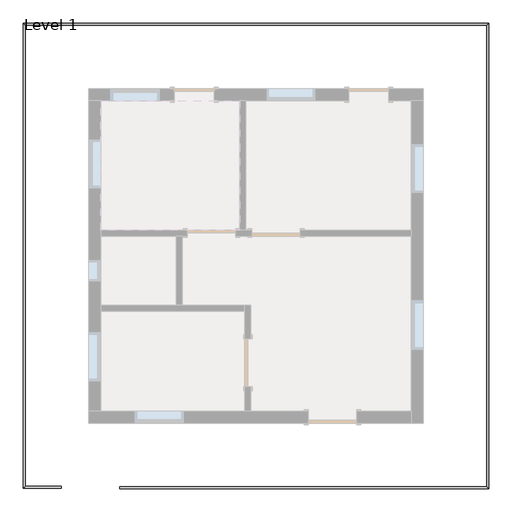
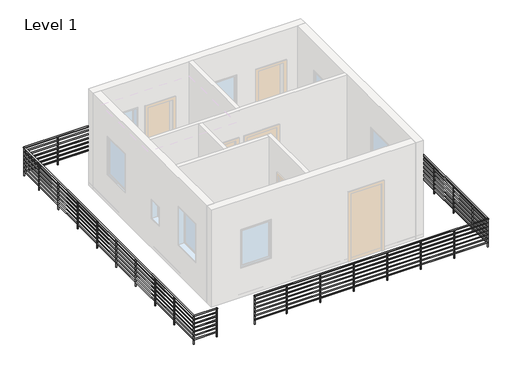
# One storey, part 2 of 2: 1 railing.
"""IFC4 building model written with IfcOpenShell, lengths in millimetres."""

from ifc_helpers import new_model, si_unit, point, frame, frame_2d, origin, origin_with_axes, place, context, project, spatial, circle_curve, ellipse_curve, trimmed, segment, composite_curve, outline, extrude, element, save
from ifc_brep_helpers import plane_surface, cylinder_surface, advanced_brep

model = new_model("IFC4")

# Units and contexts
model_context = context("Model", 3, world=origin())
ifc_project = project(units=[si_unit("LENGTHUNIT", "METRE", prefix="MILLI")], contexts=[model_context])

# Site, building, storey
site = spatial("IfcSite", under=ifc_project)
building = spatial("IfcBuilding", under=site)
storey = spatial("IfcBuildingStorey", under=building, Name="Level 1", Elevation=0.0)

# Railing
placement = place(None, origin())
element("IfcRailing", 1, ObjectType="900mm Pipe", at=placement, inside=storey, context=model_context, shape_type="SolidModel", body=[
    advanced_brep(
    [(-15823.6523905, -4811.14356, 880.0), (-15823.6523905, -4851.14356, 880.0), (-16499.9443193, -4811.14356, 880.0), (-16539.9443193, -4851.14356, 880.0), (-16499.9443193, 3906.0356469, 880.0), (-16539.9443193, 3946.0356469, 880.0), (-7776.9443193, 3906.0356469, 880.0), (-7736.9443193, 3946.0356469, 880.0), (-7776.9443193, -4816.9643531, 880.0), (-7736.9443193, -4856.9643531, 880.0), (-14716.5443193, -4816.9643531, 880.0), (-14716.5443193, -4856.9643531, 880.0)],
    [
        (0, 1, circle_curve(frame((-15823.6523905, -4831.14356, 880.0), z_axis=(1.0, 0.0, 0.0), x_axis=(0.0, -1.0, 0.0)), 20.0)),
        (1, 0, circle_curve(frame((-15823.6523905, -4831.14356, 880.0), z_axis=(1.0, 0.0, 0.0), x_axis=(0.0, -1.0, 0.0)), 20.0)),
        (0, 2),
        (2, 3, ellipse_curve(frame((-16519.9443193, -4831.14356, 880.0), z_axis=(0.7071067811865458, -0.7071067811865492, 0.0), x_axis=(0.7071067811865492, 0.7071067811865458, 0.0)), 28.2842712, 20.0)),
        (3, 1),
        (3, 2, ellipse_curve(frame((-16519.9443193, -4831.14356, 880.0), z_axis=(0.7071067811865458, -0.7071067811865492, 0.0), x_axis=(0.7071067811865492, 0.7071067811865458, 0.0)), 28.2842712, 20.0)),
        (2, 4),
        (4, 5, ellipse_curve(frame((-16519.9443193, 3926.0356469, 880.0), z_axis=(-0.7071067811865493, -0.7071067811865457, 0.0), x_axis=(0.7071067811865457, -0.7071067811865495, 0.0)), 28.2842712, 20.0)),
        (5, 3),
        (5, 4, ellipse_curve(frame((-16519.9443193, 3926.0356469, 880.0), z_axis=(-0.7071067811865493, -0.7071067811865457, 0.0), x_axis=(0.7071067811865457, -0.7071067811865495, 0.0)), 28.2842712, 20.0)),
        (4, 6),
        (6, 7, ellipse_curve(frame((-7756.9443193, 3926.0356469, 880.0), z_axis=(-0.7071067811865446, 0.7071067811865505, 0.0), x_axis=(-0.7071067811865505, -0.7071067811865445, 0.0)), 28.2842712, 20.0)),
        (7, 5),
        (7, 6, ellipse_curve(frame((-7756.9443193, 3926.0356469, 880.0), z_axis=(-0.7071067811865446, 0.7071067811865505, 0.0), x_axis=(-0.7071067811865505, -0.7071067811865445, 0.0)), 28.2842712, 20.0)),
        (6, 8),
        (8, 9, ellipse_curve(frame((-7756.9443193, -4836.9643531, 880.0), z_axis=(0.7071067811865505, 0.7071067811865446, 0.0), x_axis=(-0.7071067811865446, 0.7071067811865503, 0.0)), 28.2842712, 20.0)),
        (9, 7),
        (9, 8, ellipse_curve(frame((-7756.9443193, -4836.9643531, 880.0), z_axis=(0.7071067811865505, 0.7071067811865446, 0.0), x_axis=(-0.7071067811865446, 0.7071067811865503, 0.0)), 28.2842712, 20.0)),
        (10, 11, circle_curve(frame((-14716.5443193, -4836.9643531, 880.0), z_axis=(-1.0, 0.0, 0.0), x_axis=(0.0, -1.0, 0.0)), 20.0)),
        (11, 10, circle_curve(frame((-14716.5443193, -4836.9643531, 880.0), z_axis=(-1.0, 0.0, 0.0), x_axis=(0.0, -1.0, 0.0)), 20.0)),
        (8, 10),
        (11, 9),
    ],
    [
        plane_surface(frame((-15823.6523905, -4831.14356, 900.0), z_axis=(1.0, 0.0, 0.0), x_axis=(0.0, -1.0, 0.0))),
        cylinder_surface(frame((-15823.6523905, -4831.14356, 880.0), z_axis=(1.0, 0.0, 0.0), x_axis=(0.0, -1.0, 0.0)), 20.0),
        cylinder_surface(frame((-16519.9443193, -4831.14356, 880.0), z_axis=(0.0, -1.0, 0.0), x_axis=(-1.0, 0.0, 0.0)), 20.0),
        cylinder_surface(frame((-16519.9443193, 3926.0356469, 880.0), z_axis=(-1.0, 0.0, 0.0), x_axis=(0.0, 1.0, 0.0)), 20.0),
        cylinder_surface(frame((-7756.9443193, 3926.0356469, 880.0), z_axis=(0.0, 1.0, 0.0), x_axis=(1.0, 0.0, 0.0)), 20.0),
        plane_surface(frame((-14716.5443193, -4836.9643531, 900.0), z_axis=(-1.0, 0.0, 0.0), x_axis=(0.0, -1.0, 0.0))),
        cylinder_surface(frame((-7756.9443193, -4836.9643531, 880.0), z_axis=(1.0, 0.0, 0.0), x_axis=(0.0, -1.0, 0.0)), 20.0),
    ],
    [
        (0, [[1, 2]]),
        (1, [[-1, 3, 4, 5]]),
        (1, [[-2, -5, 6, -3]]),
        (2, [[-4, 7, 8, 9]]),
        (2, [[-6, -9, 10, -7]]),
        (3, [[-8, 11, 12, 13]]),
        (3, [[-10, -13, 14, -11]]),
        (4, [[-12, 15, 16, 17]]),
        (4, [[-14, -17, 18, -15]]),
        (5, [[19, 20]]),
        (6, [[-16, 21, -20, 22]]),
        (6, [[-18, -22, -19, -21]]),
    ],
),
    advanced_brep(
    [(-15823.6523905, -4846.14356, 760.0), (-15823.6523905, -4816.14356, 760.0), (-16534.9443193, -4846.14356, 760.0), (-16504.9443193, -4816.14356, 760.0), (-16534.9443193, 3941.0356469, 760.0), (-16504.9443193, 3911.0356469, 760.0), (-7741.9443193, 3941.0356469, 760.0), (-7771.9443193, 3911.0356469, 760.0), (-7741.9443193, -4851.9643531, 760.0), (-7771.9443193, -4821.9643531, 760.0), (-14716.5443193, -4851.9643531, 760.0), (-14716.5443193, -4821.9643531, 760.0)],
    [
        (0, 1, circle_curve(frame((-15823.6523905, -4831.14356, 760.0), z_axis=(1.0, 0.0, 0.0), x_axis=(0.0, 1.0, 0.0)), 15.0)),
        (1, 0, circle_curve(frame((-15823.6523905, -4831.14356, 760.0), z_axis=(1.0, 0.0, 0.0), x_axis=(0.0, 1.0, 0.0)), 15.0)),
        (0, 2),
        (2, 3, ellipse_curve(frame((-16519.9443193, -4831.14356, 760.0), z_axis=(0.7071067811865458, -0.7071067811865492, 0.0), x_axis=(0.7071067811865492, 0.7071067811865458, 0.0)), 21.2132034, 15.0)),
        (3, 1),
        (3, 2, ellipse_curve(frame((-16519.9443193, -4831.14356, 760.0), z_axis=(0.7071067811865458, -0.7071067811865492, 0.0), x_axis=(0.7071067811865492, 0.7071067811865458, 0.0)), 21.2132034, 15.0)),
        (2, 4),
        (4, 5, ellipse_curve(frame((-16519.9443193, 3926.0356469, 760.0), z_axis=(-0.7071067811865493, -0.7071067811865457, 0.0), x_axis=(0.7071067811865457, -0.7071067811865495, 0.0)), 21.2132034, 15.0)),
        (5, 3),
        (5, 4, ellipse_curve(frame((-16519.9443193, 3926.0356469, 760.0), z_axis=(-0.7071067811865493, -0.7071067811865457, 0.0), x_axis=(0.7071067811865457, -0.7071067811865495, 0.0)), 21.2132034, 15.0)),
        (4, 6),
        (6, 7, ellipse_curve(frame((-7756.9443193, 3926.0356469, 760.0), z_axis=(-0.7071067811865446, 0.7071067811865505, 0.0), x_axis=(-0.7071067811865505, -0.7071067811865445, 0.0)), 21.2132034, 15.0)),
        (7, 5),
        (7, 6, ellipse_curve(frame((-7756.9443193, 3926.0356469, 760.0), z_axis=(-0.7071067811865446, 0.7071067811865505, 0.0), x_axis=(-0.7071067811865505, -0.7071067811865445, 0.0)), 21.2132034, 15.0)),
        (6, 8),
        (8, 9, ellipse_curve(frame((-7756.9443193, -4836.9643531, 760.0), z_axis=(0.7071067811865505, 0.7071067811865446, 0.0), x_axis=(-0.7071067811865446, 0.7071067811865503, 0.0)), 21.2132034, 15.0)),
        (9, 7),
        (9, 8, ellipse_curve(frame((-7756.9443193, -4836.9643531, 760.0), z_axis=(0.7071067811865505, 0.7071067811865446, 0.0), x_axis=(-0.7071067811865446, 0.7071067811865503, 0.0)), 21.2132034, 15.0)),
        (10, 11, circle_curve(frame((-14716.5443193, -4836.9643531, 760.0), z_axis=(-1.0, 0.0, 0.0), x_axis=(0.0, 1.0, 0.0)), 15.0)),
        (11, 10, circle_curve(frame((-14716.5443193, -4836.9643531, 760.0), z_axis=(-1.0, 0.0, 0.0), x_axis=(0.0, 1.0, 0.0)), 15.0)),
        (8, 10),
        (11, 9),
    ],
    [
        plane_surface(frame((-15823.6523905, -4831.14356, 775.0), z_axis=(1.0, 0.0, 0.0), x_axis=(0.0, -1.0, 0.0))),
        cylinder_surface(frame((-15823.6523905, -4831.14356, 760.0), z_axis=(1.0, 0.0, 0.0), x_axis=(0.0, 1.0, 0.0)), 15.0),
        cylinder_surface(frame((-16519.9443193, -4831.14356, 760.0), z_axis=(0.0, -1.0, 0.0), x_axis=(1.0, 0.0, 0.0)), 15.0),
        cylinder_surface(frame((-16519.9443193, 3926.0356469, 760.0), z_axis=(-1.0, 0.0, 0.0), x_axis=(0.0, -1.0, 0.0)), 15.0),
        cylinder_surface(frame((-7756.9443193, 3926.0356469, 760.0), z_axis=(0.0, 1.0, 0.0), x_axis=(-1.0, 0.0, 0.0)), 15.0),
        plane_surface(frame((-14716.5443193, -4836.9643531, 775.0), z_axis=(-1.0, 0.0, 0.0), x_axis=(0.0, -1.0, 0.0))),
        cylinder_surface(frame((-7756.9443193, -4836.9643531, 760.0), z_axis=(1.0, 0.0, 0.0), x_axis=(0.0, 1.0, 0.0)), 15.0),
    ],
    [
        (0, [[1, 2]]),
        (1, [[-1, 3, 4, 5]]),
        (1, [[-2, -5, 6, -3]]),
        (2, [[-4, 7, 8, 9]]),
        (2, [[-6, -9, 10, -7]]),
        (3, [[-8, 11, 12, 13]]),
        (3, [[-10, -13, 14, -11]]),
        (4, [[-12, 15, 16, 17]]),
        (4, [[-14, -17, 18, -15]]),
        (5, [[19, 20]]),
        (6, [[-16, 21, -20, 22]]),
        (6, [[-18, -22, -19, -21]]),
    ],
),
    advanced_brep(
    [(-15823.6523905, -4846.14356, 635.0), (-15823.6523905, -4816.14356, 635.0), (-16534.9443193, -4846.14356, 635.0), (-16504.9443193, -4816.14356, 635.0), (-16534.9443193, 3941.0356469, 635.0), (-16504.9443193, 3911.0356469, 635.0), (-7741.9443193, 3941.0356469, 635.0), (-7771.9443193, 3911.0356469, 635.0), (-7741.9443193, -4851.9643531, 635.0), (-7771.9443193, -4821.9643531, 635.0), (-14716.5443193, -4851.9643531, 635.0), (-14716.5443193, -4821.9643531, 635.0)],
    [
        (0, 1, circle_curve(frame((-15823.6523905, -4831.14356, 635.0), z_axis=(1.0, 0.0, 0.0), x_axis=(0.0, 1.0, 0.0)), 15.0)),
        (1, 0, circle_curve(frame((-15823.6523905, -4831.14356, 635.0), z_axis=(1.0, 0.0, 0.0), x_axis=(0.0, 1.0, 0.0)), 15.0)),
        (0, 2),
        (2, 3, ellipse_curve(frame((-16519.9443193, -4831.14356, 635.0), z_axis=(0.7071067811865458, -0.7071067811865492, 0.0), x_axis=(0.7071067811865492, 0.7071067811865458, 0.0)), 21.2132034, 15.0)),
        (3, 1),
        (3, 2, ellipse_curve(frame((-16519.9443193, -4831.14356, 635.0), z_axis=(0.7071067811865458, -0.7071067811865492, 0.0), x_axis=(0.7071067811865492, 0.7071067811865458, 0.0)), 21.2132034, 15.0)),
        (2, 4),
        (4, 5, ellipse_curve(frame((-16519.9443193, 3926.0356469, 635.0), z_axis=(-0.7071067811865493, -0.7071067811865457, 0.0), x_axis=(0.7071067811865457, -0.7071067811865495, 0.0)), 21.2132034, 15.0)),
        (5, 3),
        (5, 4, ellipse_curve(frame((-16519.9443193, 3926.0356469, 635.0), z_axis=(-0.7071067811865493, -0.7071067811865457, 0.0), x_axis=(0.7071067811865457, -0.7071067811865495, 0.0)), 21.2132034, 15.0)),
        (4, 6),
        (6, 7, ellipse_curve(frame((-7756.9443193, 3926.0356469, 635.0), z_axis=(-0.7071067811865446, 0.7071067811865505, 0.0), x_axis=(-0.7071067811865505, -0.7071067811865445, 0.0)), 21.2132034, 15.0)),
        (7, 5),
        (7, 6, ellipse_curve(frame((-7756.9443193, 3926.0356469, 635.0), z_axis=(-0.7071067811865446, 0.7071067811865505, 0.0), x_axis=(-0.7071067811865505, -0.7071067811865445, 0.0)), 21.2132034, 15.0)),
        (6, 8),
        (8, 9, ellipse_curve(frame((-7756.9443193, -4836.9643531, 635.0), z_axis=(0.7071067811865505, 0.7071067811865446, 0.0), x_axis=(-0.7071067811865446, 0.7071067811865503, 0.0)), 21.2132034, 15.0)),
        (9, 7),
        (9, 8, ellipse_curve(frame((-7756.9443193, -4836.9643531, 635.0), z_axis=(0.7071067811865505, 0.7071067811865446, 0.0), x_axis=(-0.7071067811865446, 0.7071067811865503, 0.0)), 21.2132034, 15.0)),
        (10, 11, circle_curve(frame((-14716.5443193, -4836.9643531, 635.0), z_axis=(-1.0, 0.0, 0.0), x_axis=(0.0, 1.0, 0.0)), 15.0)),
        (11, 10, circle_curve(frame((-14716.5443193, -4836.9643531, 635.0), z_axis=(-1.0, 0.0, 0.0), x_axis=(0.0, 1.0, 0.0)), 15.0)),
        (8, 10),
        (11, 9),
    ],
    [
        plane_surface(frame((-15823.6523905, -4831.14356, 650.0), z_axis=(1.0, 0.0, 0.0), x_axis=(0.0, -1.0, 0.0))),
        cylinder_surface(frame((-15823.6523905, -4831.14356, 635.0), z_axis=(1.0, 0.0, 0.0), x_axis=(0.0, 1.0, 0.0)), 15.0),
        cylinder_surface(frame((-16519.9443193, -4831.14356, 635.0), z_axis=(0.0, -1.0, 0.0), x_axis=(1.0, 0.0, 0.0)), 15.0),
        cylinder_surface(frame((-16519.9443193, 3926.0356469, 635.0), z_axis=(-1.0, 0.0, 0.0), x_axis=(0.0, -1.0, 0.0)), 15.0),
        cylinder_surface(frame((-7756.9443193, 3926.0356469, 635.0), z_axis=(0.0, 1.0, 0.0), x_axis=(-1.0, 0.0, 0.0)), 15.0),
        plane_surface(frame((-14716.5443193, -4836.9643531, 650.0), z_axis=(-1.0, 0.0, 0.0), x_axis=(0.0, -1.0, 0.0))),
        cylinder_surface(frame((-7756.9443193, -4836.9643531, 635.0), z_axis=(1.0, 0.0, 0.0), x_axis=(0.0, 1.0, 0.0)), 15.0),
    ],
    [
        (0, [[1, 2]]),
        (1, [[-1, 3, 4, 5]]),
        (1, [[-2, -5, 6, -3]]),
        (2, [[-4, 7, 8, 9]]),
        (2, [[-6, -9, 10, -7]]),
        (3, [[-8, 11, 12, 13]]),
        (3, [[-10, -13, 14, -11]]),
        (4, [[-12, 15, 16, 17]]),
        (4, [[-14, -17, 18, -15]]),
        (5, [[19, 20]]),
        (6, [[-16, 21, -20, 22]]),
        (6, [[-18, -22, -19, -21]]),
    ],
),
    advanced_brep(
    [(-15823.6523905, -4846.14356, 510.0), (-15823.6523905, -4816.14356, 510.0), (-16534.9443193, -4846.14356, 510.0), (-16504.9443193, -4816.14356, 510.0), (-16534.9443193, 3941.0356469, 510.0), (-16504.9443193, 3911.0356469, 510.0), (-7741.9443193, 3941.0356469, 510.0), (-7771.9443193, 3911.0356469, 510.0), (-7741.9443193, -4851.9643531, 510.0), (-7771.9443193, -4821.9643531, 510.0), (-14716.5443193, -4851.9643531, 510.0), (-14716.5443193, -4821.9643531, 510.0)],
    [
        (0, 1, circle_curve(frame((-15823.6523905, -4831.14356, 510.0), z_axis=(1.0, 0.0, 0.0), x_axis=(0.0, 1.0, 0.0)), 15.0)),
        (1, 0, circle_curve(frame((-15823.6523905, -4831.14356, 510.0), z_axis=(1.0, 0.0, 0.0), x_axis=(0.0, 1.0, 0.0)), 15.0)),
        (0, 2),
        (2, 3, ellipse_curve(frame((-16519.9443193, -4831.14356, 510.0), z_axis=(0.7071067811865458, -0.7071067811865492, 0.0), x_axis=(0.7071067811865492, 0.7071067811865458, 0.0)), 21.2132034, 15.0)),
        (3, 1),
        (3, 2, ellipse_curve(frame((-16519.9443193, -4831.14356, 510.0), z_axis=(0.7071067811865458, -0.7071067811865492, 0.0), x_axis=(0.7071067811865492, 0.7071067811865458, 0.0)), 21.2132034, 15.0)),
        (2, 4),
        (4, 5, ellipse_curve(frame((-16519.9443193, 3926.0356469, 510.0), z_axis=(-0.7071067811865493, -0.7071067811865457, 0.0), x_axis=(0.7071067811865457, -0.7071067811865495, 0.0)), 21.2132034, 15.0)),
        (5, 3),
        (5, 4, ellipse_curve(frame((-16519.9443193, 3926.0356469, 510.0), z_axis=(-0.7071067811865493, -0.7071067811865457, 0.0), x_axis=(0.7071067811865457, -0.7071067811865495, 0.0)), 21.2132034, 15.0)),
        (4, 6),
        (6, 7, ellipse_curve(frame((-7756.9443193, 3926.0356469, 510.0), z_axis=(-0.7071067811865446, 0.7071067811865505, 0.0), x_axis=(-0.7071067811865505, -0.7071067811865445, 0.0)), 21.2132034, 15.0)),
        (7, 5),
        (7, 6, ellipse_curve(frame((-7756.9443193, 3926.0356469, 510.0), z_axis=(-0.7071067811865446, 0.7071067811865505, 0.0), x_axis=(-0.7071067811865505, -0.7071067811865445, 0.0)), 21.2132034, 15.0)),
        (6, 8),
        (8, 9, ellipse_curve(frame((-7756.9443193, -4836.9643531, 510.0), z_axis=(0.7071067811865505, 0.7071067811865446, 0.0), x_axis=(-0.7071067811865446, 0.7071067811865503, 0.0)), 21.2132034, 15.0)),
        (9, 7),
        (9, 8, ellipse_curve(frame((-7756.9443193, -4836.9643531, 510.0), z_axis=(0.7071067811865505, 0.7071067811865446, 0.0), x_axis=(-0.7071067811865446, 0.7071067811865503, 0.0)), 21.2132034, 15.0)),
        (10, 11, circle_curve(frame((-14716.5443193, -4836.9643531, 510.0), z_axis=(-1.0, 0.0, 0.0), x_axis=(0.0, 1.0, 0.0)), 15.0)),
        (11, 10, circle_curve(frame((-14716.5443193, -4836.9643531, 510.0), z_axis=(-1.0, 0.0, 0.0), x_axis=(0.0, 1.0, 0.0)), 15.0)),
        (8, 10),
        (11, 9),
    ],
    [
        plane_surface(frame((-15823.6523905, -4831.14356, 525.0), z_axis=(1.0, 0.0, 0.0), x_axis=(0.0, -1.0, 0.0))),
        cylinder_surface(frame((-15823.6523905, -4831.14356, 510.0), z_axis=(1.0, 0.0, 0.0), x_axis=(0.0, 1.0, 0.0)), 15.0),
        cylinder_surface(frame((-16519.9443193, -4831.14356, 510.0), z_axis=(0.0, -1.0, 0.0), x_axis=(1.0, 0.0, 0.0)), 15.0),
        cylinder_surface(frame((-16519.9443193, 3926.0356469, 510.0), z_axis=(-1.0, 0.0, 0.0), x_axis=(0.0, -1.0, 0.0)), 15.0),
        cylinder_surface(frame((-7756.9443193, 3926.0356469, 510.0), z_axis=(0.0, 1.0, 0.0), x_axis=(-1.0, 0.0, 0.0)), 15.0),
        plane_surface(frame((-14716.5443193, -4836.9643531, 525.0), z_axis=(-1.0, 0.0, 0.0), x_axis=(0.0, -1.0, 0.0))),
        cylinder_surface(frame((-7756.9443193, -4836.9643531, 510.0), z_axis=(1.0, 0.0, 0.0), x_axis=(0.0, 1.0, 0.0)), 15.0),
    ],
    [
        (0, [[1, 2]]),
        (1, [[-1, 3, 4, 5]]),
        (1, [[-2, -5, 6, -3]]),
        (2, [[-4, 7, 8, 9]]),
        (2, [[-6, -9, 10, -7]]),
        (3, [[-8, 11, 12, 13]]),
        (3, [[-10, -13, 14, -11]]),
        (4, [[-12, 15, 16, 17]]),
        (4, [[-14, -17, 18, -15]]),
        (5, [[19, 20]]),
        (6, [[-16, 21, -20, 22]]),
        (6, [[-18, -22, -19, -21]]),
    ],
),
    advanced_brep(
    [(-15823.6523905, -4846.14356, 385.0), (-15823.6523905, -4816.14356, 385.0), (-16534.9443193, -4846.14356, 385.0), (-16504.9443193, -4816.14356, 385.0), (-16534.9443193, 3941.0356469, 385.0), (-16504.9443193, 3911.0356469, 385.0), (-7741.9443193, 3941.0356469, 385.0), (-7771.9443193, 3911.0356469, 385.0), (-7741.9443193, -4851.9643531, 385.0), (-7771.9443193, -4821.9643531, 385.0), (-14716.5443193, -4851.9643531, 385.0), (-14716.5443193, -4821.9643531, 385.0)],
    [
        (0, 1, circle_curve(frame((-15823.6523905, -4831.14356, 385.0), z_axis=(1.0, 0.0, 0.0), x_axis=(0.0, 1.0, 0.0)), 15.0)),
        (1, 0, circle_curve(frame((-15823.6523905, -4831.14356, 385.0), z_axis=(1.0, 0.0, 0.0), x_axis=(0.0, 1.0, 0.0)), 15.0)),
        (0, 2),
        (2, 3, ellipse_curve(frame((-16519.9443193, -4831.14356, 385.0), z_axis=(0.7071067811865458, -0.7071067811865492, 0.0), x_axis=(0.7071067811865492, 0.7071067811865458, 0.0)), 21.2132034, 15.0)),
        (3, 1),
        (3, 2, ellipse_curve(frame((-16519.9443193, -4831.14356, 385.0), z_axis=(0.7071067811865458, -0.7071067811865492, 0.0), x_axis=(0.7071067811865492, 0.7071067811865458, 0.0)), 21.2132034, 15.0)),
        (2, 4),
        (4, 5, ellipse_curve(frame((-16519.9443193, 3926.0356469, 385.0), z_axis=(-0.7071067811865493, -0.7071067811865457, 0.0), x_axis=(0.7071067811865457, -0.7071067811865495, 0.0)), 21.2132034, 15.0)),
        (5, 3),
        (5, 4, ellipse_curve(frame((-16519.9443193, 3926.0356469, 385.0), z_axis=(-0.7071067811865493, -0.7071067811865457, 0.0), x_axis=(0.7071067811865457, -0.7071067811865495, 0.0)), 21.2132034, 15.0)),
        (4, 6),
        (6, 7, ellipse_curve(frame((-7756.9443193, 3926.0356469, 385.0), z_axis=(-0.7071067811865446, 0.7071067811865505, 0.0), x_axis=(-0.7071067811865505, -0.7071067811865445, 0.0)), 21.2132034, 15.0)),
        (7, 5),
        (7, 6, ellipse_curve(frame((-7756.9443193, 3926.0356469, 385.0), z_axis=(-0.7071067811865446, 0.7071067811865505, 0.0), x_axis=(-0.7071067811865505, -0.7071067811865445, 0.0)), 21.2132034, 15.0)),
        (6, 8),
        (8, 9, ellipse_curve(frame((-7756.9443193, -4836.9643531, 385.0), z_axis=(0.7071067811865505, 0.7071067811865446, 0.0), x_axis=(-0.7071067811865446, 0.7071067811865503, 0.0)), 21.2132034, 15.0)),
        (9, 7),
        (9, 8, ellipse_curve(frame((-7756.9443193, -4836.9643531, 385.0), z_axis=(0.7071067811865505, 0.7071067811865446, 0.0), x_axis=(-0.7071067811865446, 0.7071067811865503, 0.0)), 21.2132034, 15.0)),
        (10, 11, circle_curve(frame((-14716.5443193, -4836.9643531, 385.0), z_axis=(-1.0, 0.0, 0.0), x_axis=(0.0, 1.0, 0.0)), 15.0)),
        (11, 10, circle_curve(frame((-14716.5443193, -4836.9643531, 385.0), z_axis=(-1.0, 0.0, 0.0), x_axis=(0.0, 1.0, 0.0)), 15.0)),
        (8, 10),
        (11, 9),
    ],
    [
        plane_surface(frame((-15823.6523905, -4831.14356, 400.0), z_axis=(1.0, 0.0, 0.0), x_axis=(0.0, -1.0, 0.0))),
        cylinder_surface(frame((-15823.6523905, -4831.14356, 385.0), z_axis=(1.0, 0.0, 0.0), x_axis=(0.0, 1.0, 0.0)), 15.0),
        cylinder_surface(frame((-16519.9443193, -4831.14356, 385.0), z_axis=(0.0, -1.0, 0.0), x_axis=(1.0, 0.0, 0.0)), 15.0),
        cylinder_surface(frame((-16519.9443193, 3926.0356469, 385.0), z_axis=(-1.0, 0.0, 0.0), x_axis=(0.0, -1.0, 0.0)), 15.0),
        cylinder_surface(frame((-7756.9443193, 3926.0356469, 385.0), z_axis=(0.0, 1.0, 0.0), x_axis=(-1.0, 0.0, 0.0)), 15.0),
        plane_surface(frame((-14716.5443193, -4836.9643531, 400.0), z_axis=(-1.0, 0.0, 0.0), x_axis=(0.0, -1.0, 0.0))),
        cylinder_surface(frame((-7756.9443193, -4836.9643531, 385.0), z_axis=(1.0, 0.0, 0.0), x_axis=(0.0, 1.0, 0.0)), 15.0),
    ],
    [
        (0, [[1, 2]]),
        (1, [[-1, 3, 4, 5]]),
        (1, [[-2, -5, 6, -3]]),
        (2, [[-4, 7, 8, 9]]),
        (2, [[-6, -9, 10, -7]]),
        (3, [[-8, 11, 12, 13]]),
        (3, [[-10, -13, 14, -11]]),
        (4, [[-12, 15, 16, 17]]),
        (4, [[-14, -17, 18, -15]]),
        (5, [[19, 20]]),
        (6, [[-16, 21, -20, 22]]),
        (6, [[-18, -22, -19, -21]]),
    ],
),
    advanced_brep(
    [(-15823.6523905, -4846.14356, 260.0), (-15823.6523905, -4816.14356, 260.0), (-16534.9443193, -4846.14356, 260.0), (-16504.9443193, -4816.14356, 260.0), (-16534.9443193, 3941.0356469, 260.0), (-16504.9443193, 3911.0356469, 260.0), (-7741.9443193, 3941.0356469, 260.0), (-7771.9443193, 3911.0356469, 260.0), (-7741.9443193, -4851.9643531, 260.0), (-7771.9443193, -4821.9643531, 260.0), (-14716.5443193, -4851.9643531, 260.0), (-14716.5443193, -4821.9643531, 260.0)],
    [
        (0, 1, circle_curve(frame((-15823.6523905, -4831.14356, 260.0), z_axis=(1.0, 0.0, 0.0), x_axis=(0.0, 1.0, 0.0)), 15.0)),
        (1, 0, circle_curve(frame((-15823.6523905, -4831.14356, 260.0), z_axis=(1.0, 0.0, 0.0), x_axis=(0.0, 1.0, 0.0)), 15.0)),
        (0, 2),
        (2, 3, ellipse_curve(frame((-16519.9443193, -4831.14356, 260.0), z_axis=(0.7071067811865458, -0.7071067811865492, 0.0), x_axis=(0.7071067811865492, 0.7071067811865458, 0.0)), 21.2132034, 15.0)),
        (3, 1),
        (3, 2, ellipse_curve(frame((-16519.9443193, -4831.14356, 260.0), z_axis=(0.7071067811865458, -0.7071067811865492, 0.0), x_axis=(0.7071067811865492, 0.7071067811865458, 0.0)), 21.2132034, 15.0)),
        (2, 4),
        (4, 5, ellipse_curve(frame((-16519.9443193, 3926.0356469, 260.0), z_axis=(-0.7071067811865493, -0.7071067811865457, 0.0), x_axis=(0.7071067811865457, -0.7071067811865495, 0.0)), 21.2132034, 15.0)),
        (5, 3),
        (5, 4, ellipse_curve(frame((-16519.9443193, 3926.0356469, 260.0), z_axis=(-0.7071067811865493, -0.7071067811865457, 0.0), x_axis=(0.7071067811865457, -0.7071067811865495, 0.0)), 21.2132034, 15.0)),
        (4, 6),
        (6, 7, ellipse_curve(frame((-7756.9443193, 3926.0356469, 260.0), z_axis=(-0.7071067811865446, 0.7071067811865505, 0.0), x_axis=(-0.7071067811865505, -0.7071067811865445, 0.0)), 21.2132034, 15.0)),
        (7, 5),
        (7, 6, ellipse_curve(frame((-7756.9443193, 3926.0356469, 260.0), z_axis=(-0.7071067811865446, 0.7071067811865505, 0.0), x_axis=(-0.7071067811865505, -0.7071067811865445, 0.0)), 21.2132034, 15.0)),
        (6, 8),
        (8, 9, ellipse_curve(frame((-7756.9443193, -4836.9643531, 260.0), z_axis=(0.7071067811865505, 0.7071067811865446, 0.0), x_axis=(-0.7071067811865446, 0.7071067811865503, 0.0)), 21.2132034, 15.0)),
        (9, 7),
        (9, 8, ellipse_curve(frame((-7756.9443193, -4836.9643531, 260.0), z_axis=(0.7071067811865505, 0.7071067811865446, 0.0), x_axis=(-0.7071067811865446, 0.7071067811865503, 0.0)), 21.2132034, 15.0)),
        (10, 11, circle_curve(frame((-14716.5443193, -4836.9643531, 260.0), z_axis=(-1.0, 0.0, 0.0), x_axis=(0.0, 1.0, 0.0)), 15.0)),
        (11, 10, circle_curve(frame((-14716.5443193, -4836.9643531, 260.0), z_axis=(-1.0, 0.0, 0.0), x_axis=(0.0, 1.0, 0.0)), 15.0)),
        (8, 10),
        (11, 9),
    ],
    [
        plane_surface(frame((-15823.6523905, -4831.14356, 275.0), z_axis=(1.0, 0.0, 0.0), x_axis=(0.0, -1.0, 0.0))),
        cylinder_surface(frame((-15823.6523905, -4831.14356, 260.0), z_axis=(1.0, 0.0, 0.0), x_axis=(0.0, 1.0, 0.0)), 15.0),
        cylinder_surface(frame((-16519.9443193, -4831.14356, 260.0), z_axis=(0.0, -1.0, 0.0), x_axis=(1.0, 0.0, 0.0)), 15.0),
        cylinder_surface(frame((-16519.9443193, 3926.0356469, 260.0), z_axis=(-1.0, 0.0, 0.0), x_axis=(0.0, -1.0, 0.0)), 15.0),
        cylinder_surface(frame((-7756.9443193, 3926.0356469, 260.0), z_axis=(0.0, 1.0, 0.0), x_axis=(-1.0, 0.0, 0.0)), 15.0),
        plane_surface(frame((-14716.5443193, -4836.9643531, 275.0), z_axis=(-1.0, 0.0, 0.0), x_axis=(0.0, -1.0, 0.0))),
        cylinder_surface(frame((-7756.9443193, -4836.9643531, 260.0), z_axis=(1.0, 0.0, 0.0), x_axis=(0.0, 1.0, 0.0)), 15.0),
    ],
    [
        (0, [[1, 2]]),
        (1, [[-1, 3, 4, 5]]),
        (1, [[-2, -5, 6, -3]]),
        (2, [[-4, 7, 8, 9]]),
        (2, [[-6, -9, 10, -7]]),
        (3, [[-8, 11, 12, 13]]),
        (3, [[-10, -13, 14, -11]]),
        (4, [[-12, 15, 16, 17]]),
        (4, [[-14, -17, 18, -15]]),
        (5, [[19, 20]]),
        (6, [[-16, 21, -20, 22]]),
        (6, [[-18, -22, -19, -21]]),
    ],
),
    advanced_brep(
    [(-15823.6523905, -4846.14356, 135.0), (-15823.6523905, -4816.14356, 135.0), (-16534.9443193, -4846.14356, 135.0), (-16504.9443193, -4816.14356, 135.0), (-16534.9443193, 3941.0356469, 135.0), (-16504.9443193, 3911.0356469, 135.0), (-7741.9443193, 3941.0356469, 135.0), (-7771.9443193, 3911.0356469, 135.0), (-7741.9443193, -4851.9643531, 135.0), (-7771.9443193, -4821.9643531, 135.0), (-14716.5443193, -4851.9643531, 135.0), (-14716.5443193, -4821.9643531, 135.0)],
    [
        (0, 1, circle_curve(frame((-15823.6523905, -4831.14356, 135.0), z_axis=(1.0, 0.0, 0.0), x_axis=(0.0, 1.0, 0.0)), 15.0)),
        (1, 0, circle_curve(frame((-15823.6523905, -4831.14356, 135.0), z_axis=(1.0, 0.0, 0.0), x_axis=(0.0, 1.0, 0.0)), 15.0)),
        (0, 2),
        (2, 3, ellipse_curve(frame((-16519.9443193, -4831.14356, 135.0), z_axis=(0.7071067811865458, -0.7071067811865492, 0.0), x_axis=(0.7071067811865492, 0.7071067811865458, 0.0)), 21.2132034, 15.0)),
        (3, 1),
        (3, 2, ellipse_curve(frame((-16519.9443193, -4831.14356, 135.0), z_axis=(0.7071067811865458, -0.7071067811865492, 0.0), x_axis=(0.7071067811865492, 0.7071067811865458, 0.0)), 21.2132034, 15.0)),
        (2, 4),
        (4, 5, ellipse_curve(frame((-16519.9443193, 3926.0356469, 135.0), z_axis=(-0.7071067811865493, -0.7071067811865457, 0.0), x_axis=(0.7071067811865457, -0.7071067811865495, 0.0)), 21.2132034, 15.0)),
        (5, 3),
        (5, 4, ellipse_curve(frame((-16519.9443193, 3926.0356469, 135.0), z_axis=(-0.7071067811865493, -0.7071067811865457, 0.0), x_axis=(0.7071067811865457, -0.7071067811865495, 0.0)), 21.2132034, 15.0)),
        (4, 6),
        (6, 7, ellipse_curve(frame((-7756.9443193, 3926.0356469, 135.0), z_axis=(-0.7071067811865446, 0.7071067811865505, 0.0), x_axis=(-0.7071067811865505, -0.7071067811865445, 0.0)), 21.2132034, 15.0)),
        (7, 5),
        (7, 6, ellipse_curve(frame((-7756.9443193, 3926.0356469, 135.0), z_axis=(-0.7071067811865446, 0.7071067811865505, 0.0), x_axis=(-0.7071067811865505, -0.7071067811865445, 0.0)), 21.2132034, 15.0)),
        (6, 8),
        (8, 9, ellipse_curve(frame((-7756.9443193, -4836.9643531, 135.0), z_axis=(0.7071067811865505, 0.7071067811865446, 0.0), x_axis=(-0.7071067811865446, 0.7071067811865503, 0.0)), 21.2132034, 15.0)),
        (9, 7),
        (9, 8, ellipse_curve(frame((-7756.9443193, -4836.9643531, 135.0), z_axis=(0.7071067811865505, 0.7071067811865446, 0.0), x_axis=(-0.7071067811865446, 0.7071067811865503, 0.0)), 21.2132034, 15.0)),
        (10, 11, circle_curve(frame((-14716.5443193, -4836.9643531, 135.0), z_axis=(-1.0, 0.0, 0.0), x_axis=(0.0, 1.0, 0.0)), 15.0)),
        (11, 10, circle_curve(frame((-14716.5443193, -4836.9643531, 135.0), z_axis=(-1.0, 0.0, 0.0), x_axis=(0.0, 1.0, 0.0)), 15.0)),
        (8, 10),
        (11, 9),
    ],
    [
        plane_surface(frame((-15823.6523905, -4831.14356, 150.0), z_axis=(1.0, 0.0, 0.0), x_axis=(0.0, -1.0, 0.0))),
        cylinder_surface(frame((-15823.6523905, -4831.14356, 135.0), z_axis=(1.0, 0.0, 0.0), x_axis=(0.0, 1.0, 0.0)), 15.0),
        cylinder_surface(frame((-16519.9443193, -4831.14356, 135.0), z_axis=(0.0, -1.0, 0.0), x_axis=(1.0, 0.0, 0.0)), 15.0),
        cylinder_surface(frame((-16519.9443193, 3926.0356469, 135.0), z_axis=(-1.0, 0.0, 0.0), x_axis=(0.0, -1.0, 0.0)), 15.0),
        cylinder_surface(frame((-7756.9443193, 3926.0356469, 135.0), z_axis=(0.0, 1.0, 0.0), x_axis=(-1.0, 0.0, 0.0)), 15.0),
        plane_surface(frame((-14716.5443193, -4836.9643531, 150.0), z_axis=(-1.0, 0.0, 0.0), x_axis=(0.0, -1.0, 0.0))),
        cylinder_surface(frame((-7756.9443193, -4836.9643531, 135.0), z_axis=(1.0, 0.0, 0.0), x_axis=(0.0, 1.0, 0.0)), 15.0),
    ],
    [
        (0, [[1, 2]]),
        (1, [[-1, 3, 4, 5]]),
        (1, [[-2, -5, 6, -3]]),
        (2, [[-4, 7, 8, 9]]),
        (2, [[-6, -9, 10, -7]]),
        (3, [[-8, 11, 12, 13]]),
        (3, [[-10, -13, 14, -11]]),
        (4, [[-12, 15, 16, 17]]),
        (4, [[-14, -17, 18, -15]]),
        (5, [[19, 20]]),
        (6, [[-16, 21, -20, 22]]),
        (6, [[-18, -22, -19, -21]]),
    ],
),
    extrude(outline(composite_curve([segment(trimmed(circle_curve(frame_2d((-13756.9443193, -4836.9643531)), 12.5), [point((-13756.9443193, -4849.4643531))], [point((-13756.9443193, -4824.4643531))], False, "CARTESIAN"), True, "CONTINUOUS"), segment(trimmed(circle_curve(frame_2d((-13756.9443193, -4836.9643531)), 12.5), [point((-13756.9443193, -4824.4643531))], [point((-13756.9443193, -4849.4643531))], False, "CARTESIAN"), True, "CONTINUOUS")], self_intersect=False)), origin_with_axes(), (0.0, 0.0, 1.0), 860.0),
    extrude(outline(composite_curve([segment(trimmed(circle_curve(frame_2d((-12756.9443193, -4836.9643531)), 12.5), [point((-12756.9443193, -4849.4643531))], [point((-12756.9443193, -4824.4643531))], False, "CARTESIAN"), True, "CONTINUOUS"), segment(trimmed(circle_curve(frame_2d((-12756.9443193, -4836.9643531)), 12.5), [point((-12756.9443193, -4824.4643531))], [point((-12756.9443193, -4849.4643531))], False, "CARTESIAN"), True, "CONTINUOUS")], self_intersect=False)), origin_with_axes(), (0.0, 0.0, 1.0), 860.0),
    extrude(outline(composite_curve([segment(trimmed(circle_curve(frame_2d((-11756.9443193, -4836.9643531)), 12.5), [point((-11756.9443193, -4849.4643531))], [point((-11756.9443193, -4824.4643531))], False, "CARTESIAN"), True, "CONTINUOUS"), segment(trimmed(circle_curve(frame_2d((-11756.9443193, -4836.9643531)), 12.5), [point((-11756.9443193, -4824.4643531))], [point((-11756.9443193, -4849.4643531))], False, "CARTESIAN"), True, "CONTINUOUS")], self_intersect=False)), origin_with_axes(), (0.0, 0.0, 1.0), 860.0),
    extrude(outline(composite_curve([segment(trimmed(circle_curve(frame_2d((-10756.9443193, -4836.9643531)), 12.5), [point((-10756.9443193, -4849.4643531))], [point((-10756.9443193, -4824.4643531))], False, "CARTESIAN"), True, "CONTINUOUS"), segment(trimmed(circle_curve(frame_2d((-10756.9443193, -4836.9643531)), 12.5), [point((-10756.9443193, -4824.4643531))], [point((-10756.9443193, -4849.4643531))], False, "CARTESIAN"), True, "CONTINUOUS")], self_intersect=False)), origin_with_axes(), (0.0, 0.0, 1.0), 860.0),
    extrude(outline(composite_curve([segment(trimmed(circle_curve(frame_2d((-9756.9443193, -4836.9643531)), 12.5), [point((-9756.9443193, -4849.4643531))], [point((-9756.9443193, -4824.4643531))], False, "CARTESIAN"), True, "CONTINUOUS"), segment(trimmed(circle_curve(frame_2d((-9756.9443193, -4836.9643531)), 12.5), [point((-9756.9443193, -4824.4643531))], [point((-9756.9443193, -4849.4643531))], False, "CARTESIAN"), True, "CONTINUOUS")], self_intersect=False)), origin_with_axes(), (0.0, 0.0, 1.0), 860.0),
    extrude(outline(composite_curve([segment(trimmed(circle_curve(frame_2d((-8756.9443193, -4836.9643531)), 12.5), [point((-8756.9443193, -4849.4643531))], [point((-8756.9443193, -4824.4643531))], False, "CARTESIAN"), True, "CONTINUOUS"), segment(trimmed(circle_curve(frame_2d((-8756.9443193, -4836.9643531)), 12.5), [point((-8756.9443193, -4824.4643531))], [point((-8756.9443193, -4849.4643531))], False, "CARTESIAN"), True, "CONTINUOUS")], self_intersect=False)), origin_with_axes(), (0.0, 0.0, 1.0), 860.0),
    extrude(outline(composite_curve([segment(trimmed(circle_curve(frame_2d((-7756.9443193, -4073.9643531)), 12.5), [point((-7744.4443193, -4073.9643531))], [point((-7769.4443193, -4073.9643531))], False, "CARTESIAN"), True, "CONTINUOUS"), segment(trimmed(circle_curve(frame_2d((-7756.9443193, -4073.9643531)), 12.5), [point((-7769.4443193, -4073.9643531))], [point((-7744.4443193, -4073.9643531))], False, "CARTESIAN"), True, "CONTINUOUS")], self_intersect=False)), origin_with_axes(), (0.0, 0.0, 1.0), 860.0),
    extrude(outline(composite_curve([segment(trimmed(circle_curve(frame_2d((-7756.9443193, -3073.9643531)), 12.5), [point((-7744.4443193, -3073.9643531))], [point((-7769.4443193, -3073.9643531))], False, "CARTESIAN"), True, "CONTINUOUS"), segment(trimmed(circle_curve(frame_2d((-7756.9443193, -3073.9643531)), 12.5), [point((-7769.4443193, -3073.9643531))], [point((-7744.4443193, -3073.9643531))], False, "CARTESIAN"), True, "CONTINUOUS")], self_intersect=False)), origin_with_axes(), (0.0, 0.0, 1.0), 860.0),
    extrude(outline(composite_curve([segment(trimmed(circle_curve(frame_2d((-7756.9443193, -2073.9643531)), 12.5), [point((-7744.4443193, -2073.9643531))], [point((-7769.4443193, -2073.9643531))], False, "CARTESIAN"), True, "CONTINUOUS"), segment(trimmed(circle_curve(frame_2d((-7756.9443193, -2073.9643531)), 12.5), [point((-7769.4443193, -2073.9643531))], [point((-7744.4443193, -2073.9643531))], False, "CARTESIAN"), True, "CONTINUOUS")], self_intersect=False)), origin_with_axes(), (0.0, 0.0, 1.0), 860.0),
    extrude(outline(composite_curve([segment(trimmed(circle_curve(frame_2d((-7756.9443193, -1073.9643531)), 12.5), [point((-7744.4443193, -1073.9643531))], [point((-7769.4443193, -1073.9643531))], False, "CARTESIAN"), True, "CONTINUOUS"), segment(trimmed(circle_curve(frame_2d((-7756.9443193, -1073.9643531)), 12.5), [point((-7769.4443193, -1073.9643531))], [point((-7744.4443193, -1073.9643531))], False, "CARTESIAN"), True, "CONTINUOUS")], self_intersect=False)), origin_with_axes(), (0.0, 0.0, 1.0), 860.0),
    extrude(outline(composite_curve([segment(trimmed(circle_curve(frame_2d((-7756.9443193, -73.9643531)), 12.5), [point((-7744.4443193, -73.9643531))], [point((-7769.4443193, -73.9643531))], False, "CARTESIAN"), True, "CONTINUOUS"), segment(trimmed(circle_curve(frame_2d((-7756.9443193, -73.9643531)), 12.5), [point((-7769.4443193, -73.9643531))], [point((-7744.4443193, -73.9643531))], False, "CARTESIAN"), True, "CONTINUOUS")], self_intersect=False)), origin_with_axes(), (0.0, 0.0, 1.0), 860.0),
    extrude(outline(composite_curve([segment(trimmed(circle_curve(frame_2d((-7756.9443193, 926.0356469)), 12.5), [point((-7744.4443193, 926.0356469))], [point((-7769.4443193, 926.0356469))], False, "CARTESIAN"), True, "CONTINUOUS"), segment(trimmed(circle_curve(frame_2d((-7756.9443193, 926.0356469)), 12.5), [point((-7769.4443193, 926.0356469))], [point((-7744.4443193, 926.0356469))], False, "CARTESIAN"), True, "CONTINUOUS")], self_intersect=False)), origin_with_axes(), (0.0, 0.0, 1.0), 860.0),
    extrude(outline(composite_curve([segment(trimmed(circle_curve(frame_2d((-7756.9443193, 1926.0356469)), 12.5), [point((-7744.4443193, 1926.0356469))], [point((-7769.4443193, 1926.0356469))], False, "CARTESIAN"), True, "CONTINUOUS"), segment(trimmed(circle_curve(frame_2d((-7756.9443193, 1926.0356469)), 12.5), [point((-7769.4443193, 1926.0356469))], [point((-7744.4443193, 1926.0356469))], False, "CARTESIAN"), True, "CONTINUOUS")], self_intersect=False)), origin_with_axes(), (0.0, 0.0, 1.0), 860.0),
    extrude(outline(composite_curve([segment(trimmed(circle_curve(frame_2d((-7756.9443193, 2926.0356469)), 12.5), [point((-7744.4443193, 2926.0356469))], [point((-7769.4443193, 2926.0356469))], False, "CARTESIAN"), True, "CONTINUOUS"), segment(trimmed(circle_curve(frame_2d((-7756.9443193, 2926.0356469)), 12.5), [point((-7769.4443193, 2926.0356469))], [point((-7744.4443193, 2926.0356469))], False, "CARTESIAN"), True, "CONTINUOUS")], self_intersect=False)), origin_with_axes(), (0.0, 0.0, 1.0), 860.0),
    extrude(outline(composite_curve([segment(trimmed(circle_curve(frame_2d((-8519.9443193, 3926.0356469)), 12.5), [point((-8519.9443193, 3938.5356469))], [point((-8519.9443193, 3913.5356469))], False, "CARTESIAN"), True, "CONTINUOUS"), segment(trimmed(circle_curve(frame_2d((-8519.9443193, 3926.0356469)), 12.5), [point((-8519.9443193, 3913.5356469))], [point((-8519.9443193, 3938.5356469))], False, "CARTESIAN"), True, "CONTINUOUS")], self_intersect=False)), origin_with_axes(), (0.0, 0.0, 1.0), 860.0),
    extrude(outline(composite_curve([segment(trimmed(circle_curve(frame_2d((-9519.9443193, 3926.0356469)), 12.5), [point((-9519.9443193, 3938.5356469))], [point((-9519.9443193, 3913.5356469))], False, "CARTESIAN"), True, "CONTINUOUS"), segment(trimmed(circle_curve(frame_2d((-9519.9443193, 3926.0356469)), 12.5), [point((-9519.9443193, 3913.5356469))], [point((-9519.9443193, 3938.5356469))], False, "CARTESIAN"), True, "CONTINUOUS")], self_intersect=False)), origin_with_axes(), (0.0, 0.0, 1.0), 860.0),
    extrude(outline(composite_curve([segment(trimmed(circle_curve(frame_2d((-10519.9443193, 3926.0356469)), 12.5), [point((-10519.9443193, 3938.5356469))], [point((-10519.9443193, 3913.5356469))], False, "CARTESIAN"), True, "CONTINUOUS"), segment(trimmed(circle_curve(frame_2d((-10519.9443193, 3926.0356469)), 12.5), [point((-10519.9443193, 3913.5356469))], [point((-10519.9443193, 3938.5356469))], False, "CARTESIAN"), True, "CONTINUOUS")], self_intersect=False)), origin_with_axes(), (0.0, 0.0, 1.0), 860.0),
    extrude(outline(composite_curve([segment(trimmed(circle_curve(frame_2d((-11519.9443193, 3926.0356469)), 12.5), [point((-11519.9443193, 3938.5356469))], [point((-11519.9443193, 3913.5356469))], False, "CARTESIAN"), True, "CONTINUOUS"), segment(trimmed(circle_curve(frame_2d((-11519.9443193, 3926.0356469)), 12.5), [point((-11519.9443193, 3913.5356469))], [point((-11519.9443193, 3938.5356469))], False, "CARTESIAN"), True, "CONTINUOUS")], self_intersect=False)), origin_with_axes(), (0.0, 0.0, 1.0), 860.0),
    extrude(outline(composite_curve([segment(trimmed(circle_curve(frame_2d((-12519.9443193, 3926.0356469)), 12.5), [point((-12519.9443193, 3938.5356469))], [point((-12519.9443193, 3913.5356469))], False, "CARTESIAN"), True, "CONTINUOUS"), segment(trimmed(circle_curve(frame_2d((-12519.9443193, 3926.0356469)), 12.5), [point((-12519.9443193, 3913.5356469))], [point((-12519.9443193, 3938.5356469))], False, "CARTESIAN"), True, "CONTINUOUS")], self_intersect=False)), origin_with_axes(), (0.0, 0.0, 1.0), 860.0),
    extrude(outline(composite_curve([segment(trimmed(circle_curve(frame_2d((-13519.9443193, 3926.0356469)), 12.5), [point((-13519.9443193, 3938.5356469))], [point((-13519.9443193, 3913.5356469))], False, "CARTESIAN"), True, "CONTINUOUS"), segment(trimmed(circle_curve(frame_2d((-13519.9443193, 3926.0356469)), 12.5), [point((-13519.9443193, 3913.5356469))], [point((-13519.9443193, 3938.5356469))], False, "CARTESIAN"), True, "CONTINUOUS")], self_intersect=False)), origin_with_axes(), (0.0, 0.0, 1.0), 860.0),
    extrude(outline(composite_curve([segment(trimmed(circle_curve(frame_2d((-14519.9443193, 3926.0356469)), 12.5), [point((-14519.9443193, 3938.5356469))], [point((-14519.9443193, 3913.5356469))], False, "CARTESIAN"), True, "CONTINUOUS"), segment(trimmed(circle_curve(frame_2d((-14519.9443193, 3926.0356469)), 12.5), [point((-14519.9443193, 3913.5356469))], [point((-14519.9443193, 3938.5356469))], False, "CARTESIAN"), True, "CONTINUOUS")], self_intersect=False)), origin_with_axes(), (0.0, 0.0, 1.0), 860.0),
    extrude(outline(composite_curve([segment(trimmed(circle_curve(frame_2d((-15519.9443193, 3926.0356469)), 12.5), [point((-15519.9443193, 3938.5356469))], [point((-15519.9443193, 3913.5356469))], False, "CARTESIAN"), True, "CONTINUOUS"), segment(trimmed(circle_curve(frame_2d((-15519.9443193, 3926.0356469)), 12.5), [point((-15519.9443193, 3913.5356469))], [point((-15519.9443193, 3938.5356469))], False, "CARTESIAN"), True, "CONTINUOUS")], self_intersect=False)), origin_with_axes(), (0.0, 0.0, 1.0), 860.0),
    extrude(outline(composite_curve([segment(trimmed(circle_curve(frame_2d((-16519.9443193, 3168.85644)), 12.5), [point((-16532.4443193, 3168.85644))], [point((-16507.4443193, 3168.85644))], False, "CARTESIAN"), True, "CONTINUOUS"), segment(trimmed(circle_curve(frame_2d((-16519.9443193, 3168.85644)), 12.5), [point((-16507.4443193, 3168.85644))], [point((-16532.4443193, 3168.85644))], False, "CARTESIAN"), True, "CONTINUOUS")], self_intersect=False)), origin_with_axes(), (0.0, 0.0, 1.0), 860.0),
    extrude(outline(composite_curve([segment(trimmed(circle_curve(frame_2d((-16519.9443193, 2168.85644)), 12.5), [point((-16532.4443193, 2168.85644))], [point((-16507.4443193, 2168.85644))], False, "CARTESIAN"), True, "CONTINUOUS"), segment(trimmed(circle_curve(frame_2d((-16519.9443193, 2168.85644)), 12.5), [point((-16507.4443193, 2168.85644))], [point((-16532.4443193, 2168.85644))], False, "CARTESIAN"), True, "CONTINUOUS")], self_intersect=False)), origin_with_axes(), (0.0, 0.0, 1.0), 860.0),
    extrude(outline(composite_curve([segment(trimmed(circle_curve(frame_2d((-16519.9443193, 1168.85644)), 12.5), [point((-16532.4443193, 1168.85644))], [point((-16507.4443193, 1168.85644))], False, "CARTESIAN"), True, "CONTINUOUS"), segment(trimmed(circle_curve(frame_2d((-16519.9443193, 1168.85644)), 12.5), [point((-16507.4443193, 1168.85644))], [point((-16532.4443193, 1168.85644))], False, "CARTESIAN"), True, "CONTINUOUS")], self_intersect=False)), origin_with_axes(), (0.0, 0.0, 1.0), 860.0),
    extrude(outline(composite_curve([segment(trimmed(circle_curve(frame_2d((-16519.9443193, 168.85644)), 12.5), [point((-16532.4443193, 168.85644))], [point((-16507.4443193, 168.85644))], False, "CARTESIAN"), True, "CONTINUOUS"), segment(trimmed(circle_curve(frame_2d((-16519.9443193, 168.85644)), 12.5), [point((-16507.4443193, 168.85644))], [point((-16532.4443193, 168.85644))], False, "CARTESIAN"), True, "CONTINUOUS")], self_intersect=False)), origin_with_axes(), (0.0, 0.0, 1.0), 860.0),
    extrude(outline(composite_curve([segment(trimmed(circle_curve(frame_2d((-16519.9443193, -831.14356)), 12.5), [point((-16532.4443193, -831.14356))], [point((-16507.4443193, -831.14356))], False, "CARTESIAN"), True, "CONTINUOUS"), segment(trimmed(circle_curve(frame_2d((-16519.9443193, -831.14356)), 12.5), [point((-16507.4443193, -831.14356))], [point((-16532.4443193, -831.14356))], False, "CARTESIAN"), True, "CONTINUOUS")], self_intersect=False)), origin_with_axes(), (0.0, 0.0, 1.0), 860.0),
    extrude(outline(composite_curve([segment(trimmed(circle_curve(frame_2d((-16519.9443193, -1831.14356)), 12.5), [point((-16532.4443193, -1831.14356))], [point((-16507.4443193, -1831.14356))], False, "CARTESIAN"), True, "CONTINUOUS"), segment(trimmed(circle_curve(frame_2d((-16519.9443193, -1831.14356)), 12.5), [point((-16507.4443193, -1831.14356))], [point((-16532.4443193, -1831.14356))], False, "CARTESIAN"), True, "CONTINUOUS")], self_intersect=False)), origin_with_axes(), (0.0, 0.0, 1.0), 860.0),
    extrude(outline(composite_curve([segment(trimmed(circle_curve(frame_2d((-16519.9443193, -2831.14356)), 12.5), [point((-16532.4443193, -2831.14356))], [point((-16507.4443193, -2831.14356))], False, "CARTESIAN"), True, "CONTINUOUS"), segment(trimmed(circle_curve(frame_2d((-16519.9443193, -2831.14356)), 12.5), [point((-16507.4443193, -2831.14356))], [point((-16532.4443193, -2831.14356))], False, "CARTESIAN"), True, "CONTINUOUS")], self_intersect=False)), origin_with_axes(), (0.0, 0.0, 1.0), 860.0),
    extrude(outline(composite_curve([segment(trimmed(circle_curve(frame_2d((-16519.9443193, -3831.14356)), 12.5), [point((-16532.4443193, -3831.14356))], [point((-16507.4443193, -3831.14356))], False, "CARTESIAN"), True, "CONTINUOUS"), segment(trimmed(circle_curve(frame_2d((-16519.9443193, -3831.14356)), 12.5), [point((-16507.4443193, -3831.14356))], [point((-16532.4443193, -3831.14356))], False, "CARTESIAN"), True, "CONTINUOUS")], self_intersect=False)), origin_with_axes(), (0.0, 0.0, 1.0), 860.0),
    extrude(outline(composite_curve([segment(trimmed(circle_curve(frame_2d((-7756.9443193, -4836.9643531)), 12.5), [point((-7744.4443193, -4836.9643531))], [point((-7769.4443193, -4836.9643531))], False, "CARTESIAN"), True, "CONTINUOUS"), segment(trimmed(circle_curve(frame_2d((-7756.9443193, -4836.9643531)), 12.5), [point((-7769.4443193, -4836.9643531))], [point((-7744.4443193, -4836.9643531))], False, "CARTESIAN"), True, "CONTINUOUS")], self_intersect=False)), origin_with_axes(), (0.0, 0.0, 1.0), 860.0),
    extrude(outline(composite_curve([segment(trimmed(circle_curve(frame_2d((-7756.9443193, 3926.0356469)), 12.5), [point((-7756.9443193, 3938.5356469))], [point((-7756.9443193, 3913.5356469))], False, "CARTESIAN"), True, "CONTINUOUS"), segment(trimmed(circle_curve(frame_2d((-7756.9443193, 3926.0356469)), 12.5), [point((-7756.9443193, 3913.5356469))], [point((-7756.9443193, 3938.5356469))], False, "CARTESIAN"), True, "CONTINUOUS")], self_intersect=False)), origin_with_axes(), (0.0, 0.0, 1.0), 860.0),
    extrude(outline(composite_curve([segment(trimmed(circle_curve(frame_2d((-16519.9443193, 3926.0356469)), 12.5), [point((-16532.4443193, 3926.0356469))], [point((-16507.4443193, 3926.0356469))], False, "CARTESIAN"), True, "CONTINUOUS"), segment(trimmed(circle_curve(frame_2d((-16519.9443193, 3926.0356469)), 12.5), [point((-16507.4443193, 3926.0356469))], [point((-16532.4443193, 3926.0356469))], False, "CARTESIAN"), True, "CONTINUOUS")], self_intersect=False)), origin_with_axes(), (0.0, 0.0, 1.0), 860.0),
    extrude(outline(composite_curve([segment(trimmed(circle_curve(frame_2d((-16519.9443193, -4831.14356)), 12.5), [point((-16519.9443193, -4843.64356))], [point((-16519.9443193, -4818.64356))], False, "CARTESIAN"), True, "CONTINUOUS"), segment(trimmed(circle_curve(frame_2d((-16519.9443193, -4831.14356)), 12.5), [point((-16519.9443193, -4818.64356))], [point((-16519.9443193, -4843.64356))], False, "CARTESIAN"), True, "CONTINUOUS")], self_intersect=False)), origin_with_axes(), (0.0, 0.0, 1.0), 860.0),
    extrude(outline(composite_curve([segment(trimmed(circle_curve(frame_2d((-14704.0443193, -4836.9643531)), 12.5), [point((-14704.0443193, -4849.4643531))], [point((-14704.0443193, -4824.4643531))], False, "CARTESIAN"), True, "CONTINUOUS"), segment(trimmed(circle_curve(frame_2d((-14704.0443193, -4836.9643531)), 12.5), [point((-14704.0443193, -4824.4643531))], [point((-14704.0443193, -4849.4643531))], False, "CARTESIAN"), True, "CONTINUOUS")], self_intersect=False)), origin_with_axes(), (0.0, 0.0, 1.0), 860.0),
    extrude(outline(composite_curve([segment(trimmed(circle_curve(frame_2d((-15836.1523905, -4831.14356)), 12.5), [point((-15836.1523905, -4843.64356))], [point((-15836.1523905, -4818.64356))], False, "CARTESIAN"), True, "CONTINUOUS"), segment(trimmed(circle_curve(frame_2d((-15836.1523905, -4831.14356)), 12.5), [point((-15836.1523905, -4818.64356))], [point((-15836.1523905, -4843.64356))], False, "CARTESIAN"), True, "CONTINUOUS")], self_intersect=False)), origin_with_axes(), (0.0, 0.0, 1.0), 860.0),
])

save(model, "model.ifc")

# Revit data of these elements
# Type "900mm Pipe"
#   built-in parameter 1008612 = 0.019685 (stored number, unit not read)
#   built-in parameter 1008611 = 0.0984252 (stored number, unit not read)
#   built-in parameter 1008609 = 6.56168 (stored number, unit not read)
#   built-in parameter 1008604 = 0.19685 (stored number, unit not read)
#   built-in parameter 1008603 = 0.164042 (stored number, unit not read)
#   Railing Height = 900 mm
#   built-in parameter 1008630 = 2
#   built-in parameter 1008610 = 2
#   built-in parameter 1008605 = 1
#   built-in parameter 1008618 = M_Baluster - Round : 25mm
# Element 1 (IfcRailing, "900mm Pipe")
#   Phase Created = New Construction
